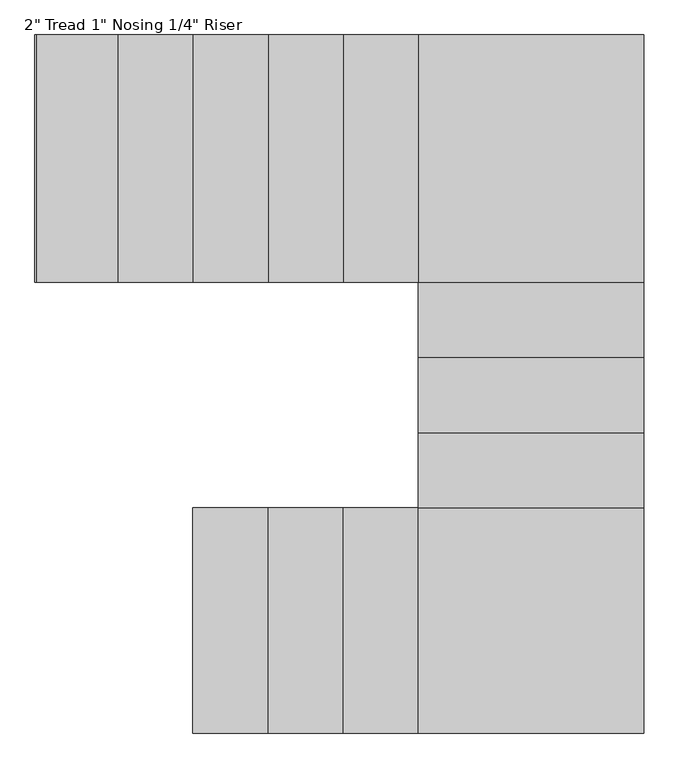
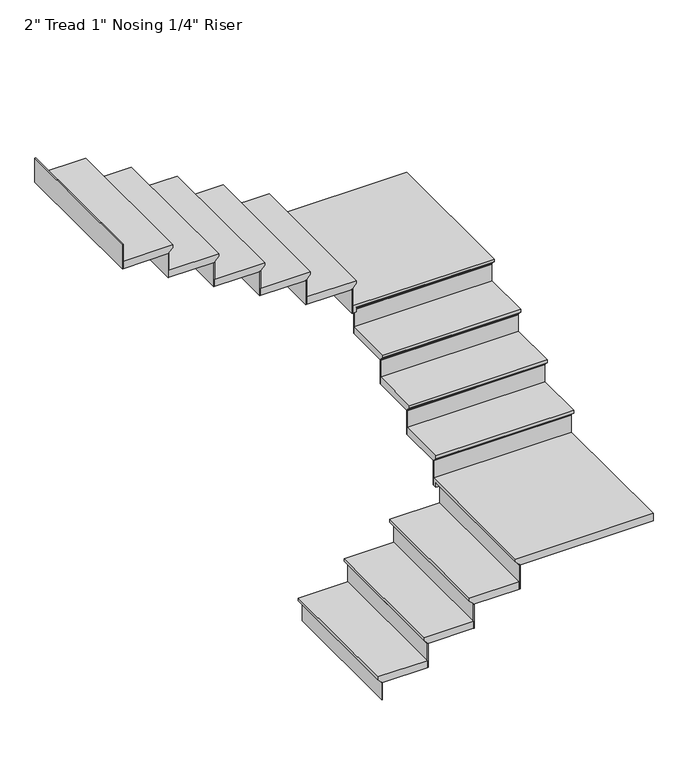
"""IFC4 building model written with IfcOpenShell, lengths in millimetres: stair flight geometry."""

from ifc_helpers import new_model, si_unit, origin, place, context, project, spatial, faceted_brep, source, transform, mapped, element, save


def stair_flight_7d6782b6(model_context):
    return source(origin(), model_context, "Body", "Brep", [
        faceted_brep([(938.5174794, -182.0870507, 150.2833333), (938.5174794, -182.0870507, 169.3333333), (938.5174794, 732.3129493, 169.3333333), (938.5174794, 732.3129493, 150.2833333), (963.9174794, -182.0870507, 124.8833333), (963.9174794, 732.3129493, 124.8833333), (1268.7174794, -182.0870507, 169.3333333), (1268.7174794, 732.3129493, 169.3333333), (963.9174794, 732.3129493, 118.5333333), (1268.7174794, 732.3129493, 118.5333333), (1268.7174794, -182.0870507, 118.5333333), (963.9174794, -182.0870507, 118.5333333)], [[[0, 1, 2, 3]], [[4, 0, 3, 5]], [[2, 1, 6, 7]], [[8, 9, 10, 11]], [[2, 7, 9, 8, 5, 3]], [[8, 11, 4, 5]], [[6, 1, 0, 4, 11, 10]], [[7, 6, 10, 9]]]),
        faceted_brep([(963.9174794, -182.0870507, 118.5333333), (963.9174794, -182.0870507, 0.0), (970.2674794, -182.0870507, 0.0), (970.2674794, -182.0870507, 118.5333333), (963.9174794, 732.3129493, 118.5333333), (970.2674794, 732.3129493, 118.5333333), (970.2674794, 732.3129493, 0.0), (963.9174794, 732.3129493, 0.0)], [[[0, 1, 2, 3]], [[4, 5, 6, 7]], [[1, 0, 4, 7]], [[2, 1, 7, 6]], [[3, 2, 6, 5]], [[0, 3, 5, 4]]]),
        faceted_brep([(1268.7174794, -182.0870507, 287.8666667), (1268.7174794, -182.0870507, 118.5333333), (1275.0674794, -182.0870507, 118.5333333), (1275.0674794, -182.0870507, 287.8666667), (1268.7174794, 732.3129493, 287.8666667), (1275.0674794, 732.3129493, 287.8666667), (1275.0674794, 732.3129493, 118.5333333), (1268.7174794, 732.3129493, 118.5333333)], [[[0, 1, 2, 3]], [[4, 5, 6, 7]], [[1, 0, 4, 7]], [[2, 1, 7, 6]], [[3, 2, 6, 5]], [[0, 3, 5, 4]]]),
        faceted_brep([(1243.3174794, 732.3129493, 338.6666667), (1243.3174794, -182.0870507, 338.6666667), (1573.5174794, -182.0870507, 338.6666667), (1573.5174794, 732.3129493, 338.6666667), (1268.7174794, 732.3129493, 287.8666667), (1573.5174794, 732.3129493, 287.8666667), (1573.5174794, -182.0870507, 287.8666667), (1268.7174794, -182.0870507, 287.8666667), (1268.7174794, 732.3129493, 294.2166667), (1243.3174794, 732.3129493, 319.6166667), (1268.7174794, -182.0870507, 294.2166667), (1243.3174794, -182.0870507, 319.6166667)], [[[0, 1, 2, 3]], [[4, 5, 6, 7]], [[0, 3, 5, 4, 8, 9]], [[4, 7, 10, 8]], [[2, 1, 11, 10, 7, 6]], [[3, 2, 6, 5]], [[11, 1, 0, 9]], [[10, 11, 9, 8]]]),
        faceted_brep([(1573.5174794, -182.0870507, 457.2), (1573.5174794, -182.0870507, 287.8666667), (1579.8674794, -182.0870507, 287.8666667), (1579.8674794, -182.0870507, 457.2), (1573.5174794, 732.3129493, 457.2), (1579.8674794, 732.3129493, 457.2), (1579.8674794, 732.3129493, 287.8666667), (1573.5174794, 732.3129493, 287.8666667)], [[[0, 1, 2, 3]], [[4, 5, 6, 7]], [[1, 0, 4, 7]], [[2, 1, 7, 6]], [[3, 2, 6, 5]], [[0, 3, 5, 4]]]),
        faceted_brep([(1548.1174794, 732.3129493, 508.0), (1548.1174794, -182.0870507, 508.0), (1878.3174794, -182.0870507, 508.0), (1878.3174794, 732.3129493, 508.0), (1573.5174794, 732.3129493, 457.2), (1878.3174794, 732.3129493, 457.2), (1878.3174794, -182.0870507, 457.2), (1573.5174794, -182.0870507, 457.2), (1573.5174794, 732.3129493, 463.55), (1548.1174794, 732.3129493, 488.95), (1573.5174794, -182.0870507, 463.55), (1548.1174794, -182.0870507, 488.95)], [[[0, 1, 2, 3]], [[4, 5, 6, 7]], [[0, 3, 5, 4, 8, 9]], [[4, 7, 10, 8]], [[2, 1, 11, 10, 7, 6]], [[3, 2, 6, 5]], [[11, 1, 0, 9]], [[10, 11, 9, 8]]]),
        faceted_brep([(1878.3174794, -182.0870507, 626.5333333), (1878.3174794, -182.0870507, 457.2), (1884.6674794, -182.0870507, 457.2), (1884.6674794, -182.0870507, 626.5333333), (1878.3174794, 732.3129493, 626.5333333), (1884.6674794, 732.3129493, 626.5333333), (1884.6674794, 732.3129493, 457.2), (1878.3174794, 732.3129493, 457.2)], [[[0, 1, 2, 3]], [[4, 5, 6, 7]], [[1, 0, 4, 7]], [[2, 1, 7, 6]], [[3, 2, 6, 5]], [[0, 3, 5, 4]]]),
        faceted_brep([(2767.3174794, -182.0870507, 677.3333333), (2767.3174794, 757.7129493, 677.3333333), (1852.9174794, 757.7129493, 677.3333333), (1852.9174794, -182.0870507, 677.3333333), (1852.9174794, 732.3129493, 626.5333333), (1852.9174794, 757.7129493, 626.5333333), (2767.3174794, 757.7129493, 626.5333333), (2767.3174794, -182.0870507, 626.5333333), (1878.3174794, -182.0870507, 626.5333333), (1878.3174794, 732.3129493, 626.5333333), (1852.9174794, 732.3129493, 658.2833333), (1852.9174794, -182.0870507, 658.2833333), (1878.3174794, 732.3129493, 632.8833333), (1878.3174794, -182.0870507, 632.8833333)], [[[0, 1, 2, 3]], [[4, 5, 6, 7, 8, 9]], [[3, 2, 5, 4, 10, 11]], [[4, 9, 12, 10]], [[9, 8, 13, 12]], [[0, 3, 11, 13, 8, 7]], [[1, 0, 7, 6]], [[2, 1, 6, 5]], [[13, 11, 10, 12]]]),
        faceted_brep([(2767.3174794, 757.7129493, 795.8666667), (2767.3174794, 757.7129493, 626.5333333), (2767.3174794, 764.0629493, 626.5333333), (2767.3174794, 764.0629493, 795.8666667), (1852.9174794, 757.7129493, 795.8666667), (1852.9174794, 764.0629493, 795.8666667), (1852.9174794, 764.0629493, 626.5333333), (1852.9174794, 757.7129493, 626.5333333)], [[[0, 1, 2, 3]], [[4, 5, 6, 7]], [[1, 0, 4, 7]], [[2, 1, 7, 6]], [[3, 2, 6, 5]], [[0, 3, 5, 4]]]),
        faceted_brep([(1852.9174794, 732.3129493, 846.6666667), (2767.3174794, 732.3129493, 846.6666667), (2767.3174794, 1062.5129493, 846.6666667), (1852.9174794, 1062.5129493, 846.6666667), (1852.9174794, 757.7129493, 795.8666667), (1852.9174794, 1062.5129493, 795.8666667), (2767.3174794, 1062.5129493, 795.8666667), (2767.3174794, 757.7129493, 795.8666667), (1852.9174794, 757.7129493, 802.2166667), (1852.9174794, 732.3129493, 827.6166667), (2767.3174794, 757.7129493, 802.2166667), (2767.3174794, 732.3129493, 827.6166667)], [[[0, 1, 2, 3]], [[4, 5, 6, 7]], [[0, 3, 5, 4, 8, 9]], [[4, 7, 10, 8]], [[2, 1, 11, 10, 7, 6]], [[3, 2, 6, 5]], [[11, 1, 0, 9]], [[10, 11, 9, 8]]]),
        faceted_brep([(2767.3174794, 1062.5129493, 965.2), (2767.3174794, 1062.5129493, 795.8666667), (2767.3174794, 1068.8629493, 795.8666667), (2767.3174794, 1068.8629493, 965.2), (1852.9174794, 1062.5129493, 965.2), (1852.9174794, 1068.8629493, 965.2), (1852.9174794, 1068.8629493, 795.8666667), (1852.9174794, 1062.5129493, 795.8666667)], [[[0, 1, 2, 3]], [[4, 5, 6, 7]], [[1, 0, 4, 7]], [[2, 1, 7, 6]], [[3, 2, 6, 5]], [[0, 3, 5, 4]]]),
        faceted_brep([(1852.9174794, 1037.1129493, 1016.0), (2767.3174794, 1037.1129493, 1016.0), (2767.3174794, 1367.3129493, 1016.0), (1852.9174794, 1367.3129493, 1016.0), (1852.9174794, 1062.5129493, 965.2), (1852.9174794, 1367.3129493, 965.2), (2767.3174794, 1367.3129493, 965.2), (2767.3174794, 1062.5129493, 965.2), (1852.9174794, 1062.5129493, 971.55), (1852.9174794, 1037.1129493, 996.95), (2767.3174794, 1062.5129493, 971.55), (2767.3174794, 1037.1129493, 996.95)], [[[0, 1, 2, 3]], [[4, 5, 6, 7]], [[0, 3, 5, 4, 8, 9]], [[4, 7, 10, 8]], [[2, 1, 11, 10, 7, 6]], [[3, 2, 6, 5]], [[11, 1, 0, 9]], [[10, 11, 9, 8]]]),
        faceted_brep([(2767.3174794, 1367.3129493, 1134.5333333), (2767.3174794, 1367.3129493, 965.2), (2767.3174794, 1373.6629493, 965.2), (2767.3174794, 1373.6629493, 1134.5333333), (1852.9174794, 1367.3129493, 1134.5333333), (1852.9174794, 1373.6629493, 1134.5333333), (1852.9174794, 1373.6629493, 965.2), (1852.9174794, 1367.3129493, 965.2)], [[[0, 1, 2, 3]], [[4, 5, 6, 7]], [[1, 0, 4, 7]], [[2, 1, 7, 6]], [[3, 2, 6, 5]], [[0, 3, 5, 4]]]),
        faceted_brep([(1852.9174794, 1341.9129493, 1185.3333333), (2767.3174794, 1341.9129493, 1185.3333333), (2767.3174794, 1672.1129493, 1185.3333333), (1852.9174794, 1672.1129493, 1185.3333333), (1852.9174794, 1367.3129493, 1134.5333333), (1852.9174794, 1672.1129493, 1134.5333333), (2767.3174794, 1672.1129493, 1134.5333333), (2767.3174794, 1367.3129493, 1134.5333333), (1852.9174794, 1367.3129493, 1140.8833333), (1852.9174794, 1341.9129493, 1166.2833333), (2767.3174794, 1367.3129493, 1140.8833333), (2767.3174794, 1341.9129493, 1166.2833333)], [[[0, 1, 2, 3]], [[4, 5, 6, 7]], [[0, 3, 5, 4, 8, 9]], [[4, 7, 10, 8]], [[2, 1, 11, 10, 7, 6]], [[3, 2, 6, 5]], [[11, 1, 0, 9]], [[10, 11, 9, 8]]]),
        faceted_brep([(2767.3174794, 1672.1129493, 1303.8666667), (2767.3174794, 1672.1129493, 1134.5333333), (2767.3174794, 1678.4629493, 1134.5333333), (2767.3174794, 1678.4629493, 1303.8666667), (1852.9174794, 1672.1129493, 1303.8666667), (1852.9174794, 1678.4629493, 1303.8666667), (1852.9174794, 1678.4629493, 1134.5333333), (1852.9174794, 1672.1129493, 1134.5333333)], [[[0, 1, 2, 3]], [[4, 5, 6, 7]], [[1, 0, 4, 7]], [[2, 1, 7, 6]], [[3, 2, 6, 5]], [[0, 3, 5, 4]]]),
        faceted_brep([(2767.3174794, 2650.0129493, 1354.6666667), (1827.5174794, 2650.0129493, 1354.6666667), (1827.5174794, 1646.7129493, 1354.6666667), (2767.3174794, 1646.7129493, 1354.6666667), (1852.9174794, 1646.7129493, 1303.8666667), (1827.5174794, 1646.7129493, 1303.8666667), (1827.5174794, 2650.0129493, 1303.8666667), (2767.3174794, 2650.0129493, 1303.8666667), (2767.3174794, 1672.1129493, 1303.8666667), (1852.9174794, 1672.1129493, 1303.8666667), (1852.9174794, 1646.7129493, 1335.6166667), (2767.3174794, 1646.7129493, 1335.6166667), (1852.9174794, 1672.1129493, 1310.2166667), (2767.3174794, 1672.1129493, 1310.2166667)], [[[0, 1, 2, 3]], [[4, 5, 6, 7, 8, 9]], [[3, 2, 5, 4, 10, 11]], [[4, 9, 12, 10]], [[9, 8, 13, 12]], [[0, 3, 11, 13, 8, 7]], [[1, 0, 7, 6]], [[2, 1, 6, 5]], [[13, 11, 10, 12]]]),
        faceted_brep([(1827.5174794, 2650.0129493, 1473.2), (1827.5174794, 2650.0129493, 1303.8666667), (1821.1674794, 2650.0129493, 1303.8666667), (1821.1674794, 2650.0129493, 1473.2), (1827.5174794, 1646.7129493, 1473.2), (1821.1674794, 1646.7129493, 1473.2), (1821.1674794, 1646.7129493, 1303.8666667), (1827.5174794, 1646.7129493, 1303.8666667)], [[[0, 1, 2, 3]], [[4, 5, 6, 7]], [[1, 0, 4, 7]], [[2, 1, 7, 6]], [[3, 2, 6, 5]], [[0, 3, 5, 4]]]),
        faceted_brep([(1852.9174794, 1646.7129493, 1524.0), (1852.9174794, 2650.0129493, 1524.0), (1522.7174794, 2650.0129493, 1524.0), (1522.7174794, 1646.7129493, 1524.0), (1827.5174794, 1646.7129493, 1473.2), (1522.7174794, 1646.7129493, 1473.2), (1522.7174794, 2650.0129493, 1473.2), (1827.5174794, 2650.0129493, 1473.2), (1827.5174794, 1646.7129493, 1479.55), (1852.9174794, 1646.7129493, 1504.95), (1827.5174794, 2650.0129493, 1479.55), (1852.9174794, 2650.0129493, 1504.95)], [[[0, 1, 2, 3]], [[4, 5, 6, 7]], [[0, 3, 5, 4, 8, 9]], [[4, 7, 10, 8]], [[2, 1, 11, 10, 7, 6]], [[3, 2, 6, 5]], [[11, 1, 0, 9]], [[10, 11, 9, 8]]]),
        faceted_brep([(1522.7174794, 2650.0129493, 1642.5333333), (1522.7174794, 2650.0129493, 1473.2), (1516.3674794, 2650.0129493, 1473.2), (1516.3674794, 2650.0129493, 1642.5333333), (1522.7174794, 1646.7129493, 1642.5333333), (1516.3674794, 1646.7129493, 1642.5333333), (1516.3674794, 1646.7129493, 1473.2), (1522.7174794, 1646.7129493, 1473.2)], [[[0, 1, 2, 3]], [[4, 5, 6, 7]], [[1, 0, 4, 7]], [[2, 1, 7, 6]], [[3, 2, 6, 5]], [[0, 3, 5, 4]]]),
        faceted_brep([(1548.1174794, 1646.7129493, 1693.3333333), (1548.1174794, 2650.0129493, 1693.3333333), (1217.9174794, 2650.0129493, 1693.3333333), (1217.9174794, 1646.7129493, 1693.3333333), (1522.7174794, 1646.7129493, 1642.5333333), (1217.9174794, 1646.7129493, 1642.5333333), (1217.9174794, 2650.0129493, 1642.5333333), (1522.7174794, 2650.0129493, 1642.5333333), (1522.7174794, 1646.7129493, 1648.8833333), (1548.1174794, 1646.7129493, 1674.2833333), (1522.7174794, 2650.0129493, 1648.8833333), (1548.1174794, 2650.0129493, 1674.2833333)], [[[0, 1, 2, 3]], [[4, 5, 6, 7]], [[0, 3, 5, 4, 8, 9]], [[4, 7, 10, 8]], [[2, 1, 11, 10, 7, 6]], [[3, 2, 6, 5]], [[11, 1, 0, 9]], [[10, 11, 9, 8]]]),
        faceted_brep([(1217.9174794, 2650.0129493, 1811.8666667), (1217.9174794, 2650.0129493, 1642.5333333), (1211.5674794, 2650.0129493, 1642.5333333), (1211.5674794, 2650.0129493, 1811.8666667), (1217.9174794, 1646.7129493, 1811.8666667), (1211.5674794, 1646.7129493, 1811.8666667), (1211.5674794, 1646.7129493, 1642.5333333), (1217.9174794, 1646.7129493, 1642.5333333)], [[[0, 1, 2, 3]], [[4, 5, 6, 7]], [[1, 0, 4, 7]], [[2, 1, 7, 6]], [[3, 2, 6, 5]], [[0, 3, 5, 4]]]),
        faceted_brep([(1243.3174794, 1646.7129493, 1862.6666667), (1243.3174794, 2650.0129493, 1862.6666667), (913.1174794, 2650.0129493, 1862.6666667), (913.1174794, 1646.7129493, 1862.6666667), (1217.9174794, 1646.7129493, 1811.8666667), (913.1174794, 1646.7129493, 1811.8666667), (913.1174794, 2650.0129493, 1811.8666667), (1217.9174794, 2650.0129493, 1811.8666667), (1217.9174794, 1646.7129493, 1818.2166667), (1243.3174794, 1646.7129493, 1843.6166667), (1217.9174794, 2650.0129493, 1818.2166667), (1243.3174794, 2650.0129493, 1843.6166667)], [[[0, 1, 2, 3]], [[4, 5, 6, 7]], [[0, 3, 5, 4, 8, 9]], [[4, 7, 10, 8]], [[2, 1, 11, 10, 7, 6]], [[3, 2, 6, 5]], [[11, 1, 0, 9]], [[10, 11, 9, 8]]]),
        faceted_brep([(913.1174794, 2650.0129493, 1981.2), (913.1174794, 2650.0129493, 1811.8666667), (906.7674794, 2650.0129493, 1811.8666667), (906.7674794, 2650.0129493, 1981.2), (913.1174794, 1646.7129493, 1981.2), (906.7674794, 1646.7129493, 1981.2), (906.7674794, 1646.7129493, 1811.8666667), (913.1174794, 1646.7129493, 1811.8666667)], [[[0, 1, 2, 3]], [[4, 5, 6, 7]], [[1, 0, 4, 7]], [[2, 1, 7, 6]], [[3, 2, 6, 5]], [[0, 3, 5, 4]]]),
        faceted_brep([(938.5174794, 1646.7129493, 2032.0), (938.5174794, 2650.0129493, 2032.0), (608.3174794, 2650.0129493, 2032.0), (608.3174794, 1646.7129493, 2032.0), (913.1174794, 1646.7129493, 1981.2), (608.3174794, 1646.7129493, 1981.2), (608.3174794, 2650.0129493, 1981.2), (913.1174794, 2650.0129493, 1981.2), (913.1174794, 1646.7129493, 1987.55), (938.5174794, 1646.7129493, 2012.95), (913.1174794, 2650.0129493, 1987.55), (938.5174794, 2650.0129493, 2012.95)], [[[0, 1, 2, 3]], [[4, 5, 6, 7]], [[0, 3, 5, 4, 8, 9]], [[4, 7, 10, 8]], [[2, 1, 11, 10, 7, 6]], [[3, 2, 6, 5]], [[11, 1, 0, 9]], [[10, 11, 9, 8]]]),
        faceted_brep([(608.3174794, 2650.0129493, 2150.5333333), (608.3174794, 2650.0129493, 1981.2), (601.9674794, 2650.0129493, 1981.2), (601.9674794, 2650.0129493, 2150.5333333), (608.3174794, 1646.7129493, 2150.5333333), (601.9674794, 1646.7129493, 2150.5333333), (601.9674794, 1646.7129493, 1981.2), (608.3174794, 1646.7129493, 1981.2)], [[[0, 1, 2, 3]], [[4, 5, 6, 7]], [[1, 0, 4, 7]], [[2, 1, 7, 6]], [[3, 2, 6, 5]], [[0, 3, 5, 4]]]),
        faceted_brep([(303.5174794, 2650.0129493, 2319.8666667), (303.5174794, 2650.0129493, 2150.5333333), (297.1674794, 2650.0129493, 2150.5333333), (297.1674794, 2650.0129493, 2319.8666667), (303.5174794, 1646.7129493, 2319.8666667), (297.1674794, 1646.7129493, 2319.8666667), (297.1674794, 1646.7129493, 2150.5333333), (303.5174794, 1646.7129493, 2150.5333333)], [[[0, 1, 2, 3]], [[4, 5, 6, 7]], [[1, 0, 4, 7]], [[2, 1, 7, 6]], [[3, 2, 6, 5]], [[0, 3, 5, 4]]]),
        faceted_brep([(633.7174794, 1646.7129493, 2201.3333333), (633.7174794, 2650.0129493, 2201.3333333), (303.5174794, 2650.0129493, 2201.3333333), (303.5174794, 1646.7129493, 2201.3333333), (608.3174794, 1646.7129493, 2150.5333333), (303.5174794, 1646.7129493, 2150.5333333), (303.5174794, 2650.0129493, 2150.5333333), (608.3174794, 2650.0129493, 2150.5333333), (608.3174794, 1646.7129493, 2156.8833333), (633.7174794, 1646.7129493, 2182.2833333), (608.3174794, 2650.0129493, 2156.8833333), (633.7174794, 2650.0129493, 2182.2833333)], [[[0, 1, 2, 3]], [[4, 5, 6, 7]], [[0, 3, 5, 4, 8, 9]], [[4, 7, 10, 8]], [[2, 1, 11, 10, 7, 6]], [[3, 2, 6, 5]], [[11, 1, 0, 9]], [[10, 11, 9, 8]]]),
    ])


if __name__ == "__main__":
    model = new_model("IFC4")
    model_context = context("Model", 3, world=origin())
    ifc_project = project(units=[si_unit("LENGTHUNIT", "METRE", prefix="MILLI")], contexts=[model_context])
    site = spatial("IfcSite", under=ifc_project)
    building = spatial("IfcBuilding", under=site)
    placement = place(None, origin())
    stair_flight_shape = stair_flight_7d6782b6(model_context)
    element("IfcStairFlight", 1, ObjectType="2\" Tread 1\" Nosing 1/4\" Riser", at=placement, inside=building, context=model_context, shape_type="MappedRepresentation", body=[
        mapped(stair_flight_shape, transform((0.0, 0.0, 0.0), x_axis=(1.0, 0.0, 0.0), y_axis=(0.0, 1.0, 0.0), z_axis=(0.0, 0.0, 1.0))),
    ])
    save(model, "model.ifc")
